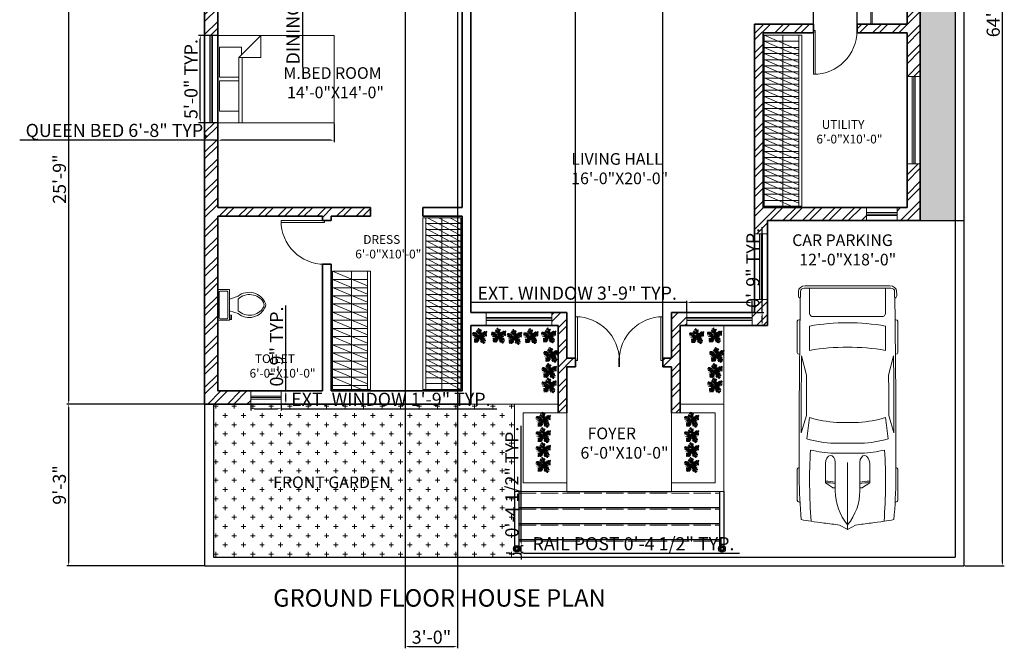
# Model space of a CAD drawing. Units: inches. Extents: x 108 to 883, y 608 to 1524.
# Tile 1 of 4: x 108 to 785, y 608 to 1040. Entities that reach past the tile are written whole.
import ezdxf

# ---------------------------------------------------------------- set-up
doc = ezdxf.new("R2010")
doc.units = ezdxf.units.IN
doc.linetypes.add('ACAD_ISO02W100', pattern=[15, 12, -3])
for name, color, linetype, lineweight in [('A-ANNO-DIMS', 2, 'Continuous', 18), ('A-ANNO-TEXT', 7, 'Continuous', 25), ('A-AREA-IDEN', 7, 'Continuous', 18), ('A-DOOR', 4, 'Continuous', 18), ('A-FLOR-CASE', 9, 'Continuous', 18), ('A-FLOR-CASE-HIDN', 9, 'ACAD_ISO02W100', 13), ('A-FLOR-CASE-PATT', 252, 'Continuous', 13), ('A-FLOR-FIXT', 9, 'Continuous', 18), ('A-FLOR-STRS', 7, 'Continuous', 25), ('A-FLOR-STRS-HIDN', 8, 'ACAD_ISO02W100', 13), ('A-FURN', 8, 'Continuous', 18), ('A-WALL', 7, 'Continuous', 35), ('A-WALL-PATT', 252, 'Continuous', 13), ('C-PKNG-VEHI', 8, 'Continuous', 13), ('C-PROP', 7, 'Continuous', 25), ('L-PLNT', 94, 'Continuous', 13), ('L-PLNT-BEDS', 94, 'Continuous', 18)]:
    doc.layers.add(name, color=color, linetype=linetype, lineweight=lineweight)
doc.layers.add('A-GLAZ', color=244, linetype='Continuous', lineweight=18, true_color=0x991b1e)
doc.layers.add('L-PLNT-PATT', color=116, linetype='Continuous', lineweight=13, true_color=0x136734)
doc.styles.get("Standard").update_dxf_attribs({"font": 'arial.ttf'})
doc.dimstyles.new('ISO-25', dxfattribs={"dimtxt": 9, "dimasz": 2.5, "dimexe": 1.25, "dimexo": 0.625, "dimtad": 1, "dimlunit": 3, "dimtxsty": 'Standard', "dimcen": 2.5, "dimadec": 0, "dimazin": 0, "dimtfac": 1, "dimtmove": 0, "dimatfit": 3, "dimfxl": 1, "dimarcsym": 0})

# ---------------------------------------------------------------- blocks, each defined once
blk = doc.blocks.new('*U2')
for p, q in [((0, 0), (0, -6)), ((40, 0), (40, -6))]:
    blk.add_line(p, q)
blk.add_lwpolyline([(0, 0), (0, 40), (1.75, 40), (1.75, 0)], close=True)
blk.add_arc((0, 0), 40, 0, 90)
blk = doc.blocks.new('*U4')
for p, q in [((0, 0), (0, -6)), ((-40, 0), (-40, -6))]:
    blk.add_line(p, q)
blk.add_lwpolyline([(0, 0), (0, 40), (-1.75, 40), (-1.75, 0)], close=True)
blk.add_arc((0, 0), 40, 90, 180)
blk = doc.blocks.new('*U7')
for p, q in [((46.55, 38.89), (22.35, 38.89)), ((136.7, 38.89), (160.9, 38.89)), ((21.1, 37.41), (21.1, 36.83)), ((47.8, 37.39), (47.8, 37.41)), ((70.03, 31.54), (86.41, 29.35)), ((87.99, 31.87), (74.76, 35.92)), ((134.31, 35.6), (119.29, 31.78)), ((135.45, 37.07), (135.45, 37.41)), ((162.15, 37.41), (162.15, 36.77)), ((186.47, -33.5), (186.47, 33.5)), ((188.4, -32.76), (188.4, 32.76)), ((138.42, 29.35), (157.25, 29.35)), ((164.52, 26.39), (164.52, -26.39)), ((186.47, 29.35), (167.01, 29.35)), ((32.27, 11.63), (36.13, 17.17)), ((36.13, 17.17), (50.94, 17.17)), ((29.77, 9.51), (51.68, 9.51)), ((32.12, 9.51), (32.12, 11.15)), ((58.92, -10.77), (58.92, 10.77)), ((66.55, -10.53), (66.55, 10.53)), ((82.74, 8.5), (82.74, -8.5)), ((186.47, -10.53), (186.47, 10.53)), ((3.27, 6.13), (0.1, 0.41)), ((0, 0), (51.68, 0)), ((0.1, -0.41), (3.27, -6.13)), ((29.77, -9.51), (51.68, -9.51)), ((32.12, -9.51), (32.12, -11.15)), ((32.27, -11.63), (36.13, -17.17)), ((36.13, -17.17), (50.94, -17.17)), ((86.41, -29.35), (70.03, -31.54)), ((157.25, -29.35), (138.42, -29.35)), ((167.01, -29.35), (186.47, -29.35)), ((21.1, -37.41), (21.1, -36.83)), ((47.8, -37.39), (47.8, -37.41)), ((87.99, -31.87), (74.76, -35.92)), ((134.31, -35.6), (119.29, -31.78)), ((135.45, -37.07), (135.45, -37.41)), ((162.15, -37.41), (162.15, -36.77)), ((46.55, -38.89), (22.35, -38.89)), ((136.7, -38.89), (160.9, -38.89))]:
    blk.add_line(p, q)
for centre, major_axis, ratio, start_param, end_param in [((22.35, 37.41), (0, -1.48), 0.842304, 3.141593, 4.712389), ((46.55, 37.41), (0, 1.48), 0.842304, -1.570796, 0), ((136.7, 37.41), (0, -1.48), 0.842304, 3.141593, 4.712389), ((160.9, 37.41), (0, 1.48), 0.842304, -1.570796, 0), ((266.03, -27.52), (0, 313.31), 0.842304, 1.367076, 1.39176), ((41.19, -490.86), (0, 528.23), 0.842304, 0.00281, 0.075598), ((64.48, -10555.62), (0, 10593.03), 0.842304, -0.013397, 0.002797), ((135.29, 5.39), (0, 81.77), 0.842304, 1.245306, 1.50788), ((64.48, -10555.62), (0, -10591.55), 0.842304, 3.133765, 3.140441), ((95.79, -3666.35), (0, -3698.24), 0.842304, 3.134049, 3.144098), ((180.63, 35.84), (0, 2.22), 0.842304, -0.013017, 1.249894), ((64.48, -10556.36), (0, 10595.31), 0.842304, -0.013397, -0.013017), ((183.98, 33.5), (0, -2.96), 0.842304, 1.570796, 3.128196), ((183.98, 32.76), (0, -5.25), 0.842304, 1.570796, 3.128196), ((259.18, -27.52), (0, -305.3), 0.842304, 4.528606, 4.561838), ((37.47, -593.96), (0, -623.33), 0.842304, 3.096046, 3.200911), ((134.4, 5.39), (0, -89.78), 0.842304, 4.449482, 4.652344), ((149.6, 2.8), (0, -79.58), 0.842304, 4.372215, 4.640744), ((17.08, 0), (0, 147.02), 0.842304, 4.511394, 4.913384), ((35.91, 0), (0, 147.02), 0.842304, 4.511394, 4.913384), ((167.01, 26.39), (0, 2.96), 0.842304, 0, 1.570796), ((-204.49, 52.4), (0, -250.96), 0.842304, 1.385369, 1.434372), ((13.04, 17.01), (0, 27.42), 0.842304, 4.435146, 4.718221), ((14.2, 17.01), (0, 27.42), 0.842304, 4.435146, 4.718221), ((50.79, 13.34), (6.34, -0.36), 0.603834, -1.395552, 1.581315), ((29.77, -46.66), (0, 56.17), 0.842304, 0, 0.590319), ((32.75, 11.15), (0, 0.74), 0.842304, 0.879714, 1.570796), ((0.62, 0), (0, -0.74), 0.842304, 4.131459, 5.293319), ((-204.49, -52.4), (0, 250.96), 0.842304, -1.434372, -1.385369), ((29.77, 46.66), (0, 56.17), 0.842304, 2.551274, 3.141593), ((32.75, -11.15), (0, -0.74), 0.842304, 4.712389, 5.403472), ((13.04, -17.01), (0, -27.42), 0.842304, 1.564964, 1.848039), ((14.2, -17.01), (0, -27.42), 0.842304, 1.564964, 1.848039), ((134.4, -5.39), (0, -89.78), 0.842304, -1.510751, -1.307889), ((135.29, -5.39), (0, -81.77), 0.842304, -1.50788, -1.245306), ((149.6, -2.8), (0, -79.58), 0.842304, -1.499151, -1.230623), ((259.18, 27.52), (0, 305.3), 0.842304, 1.721348, 1.754579), ((266.03, 27.52), (0, 313.31), 0.842304, 1.749832, 1.774517), ((37.47, 593.96), (0, -623.33), 0.842304, -0.059319, 0.045547), ((167.01, -26.39), (0, -2.96), 0.842304, 4.712389, 6.283185), ((41.19, 490.86), (0, -528.23), 0.842304, -0.075598, -0.00281), ((22.35, -37.41), (0, 1.48), 0.842304, 1.570796, 3.141593), ((64.48, 10555.62), (0, 10593.03), 0.842304, 3.138796, 3.15499), ((46.55, -37.41), (0, -1.48), 0.842304, 0, 1.570796), ((64.48, 10555.62), (0, -10591.55), 0.842304, 0.001152, 0.007828), ((95.79, 3666.35), (0, -3698.24), 0.842304, -0.002505, 0.007544), ((136.7, -37.41), (0, -1.48), 0.842304, -1.570796, 0), ((160.9, -37.41), (0, 1.48), 0.842304, 3.141593, 4.712389), ((180.63, -35.84), (0, -2.22), 0.842304, -1.249894, 0.013017), ((64.48, 10556.36), (0, 10595.31), 0.842304, 3.15461, 3.15499), ((183.98, -33.5), (0, 2.96), 0.842304, 3.15499, 4.712389), ((183.98, -32.76), (0, -5.25), 0.842304, 0.013397, 1.570796)]:
    blk.add_ellipse(centre, major_axis=major_axis, ratio=ratio, start_param=start_param, end_param=end_param)
at = {"extrusion": (0, 0, -1)}
blk.add_ellipse((50.79, -13.34), major_axis=(6.34, 0.36), ratio=0.603834, start_param=-1.395552, end_param=1.581315, dxfattribs=at)
blk = doc.blocks.new('*U9')
for p, q in [((9.5, -6), (9.5, -2)), ((-10, -8.5), (-8, -8.5)), ((-10, -9.5), (-10, -8.5)), ((-7, -9.5), (-10, -9.5)), ((-8, -8.5), (-8, -8)), ((-7, -8), (-7, -9.5)), ((-4, -8), (-6, -14)), ((4, -8), (6, -14)), ((4, -14), (-4, -14))]:
    blk.add_line(p, q)
blk.add_lwpolyline([(10.5, -8), (10.5, 0), (-10.5, 0), (-10.5, -8)], close=True)
for points in [[(-9.5, -2), (-9.5, -6)], [(8.5, -1), (-8.5, -1)], [(-8.5, -7), (8.5, -7)]]:
    blk.add_lwpolyline(points)
for centre, radius, start, end in [((-8.62, -1.88), 0.884, 81.8699, 188.1301), ((-8.62, -6.12), 0.884, 171.8699, 278.1301), ((8.62, -1.88), 0.884, 351.8699, 98.1301), ((8.62, -6.12), 0.884, 261.8699, 8.1301), ((3.52, -21.58), 12.17, 141.46911, 247.97143), ((4.2, -21.82), 11.33, 136.36773, 238.94682), ((-3.52, -21.58), 12.17, 292.02843, 38.53071), ((-4.2, -21.82), 11.33, 301.05301, 43.63209), ((0, -27.88), 4, 245.73182, 294.26817), ((0, -29), 4, 254.86053, 285.13947)]:
    blk.add_arc(centre, radius, start, end)
blk = doc.blocks.new('Bed - Queen')
for p, q in [((0, -80.00003), (0, 0)), ((0, 0), (59.99999, 0)), ((59.99999, 0), (59.99999, -80.00003)), ((7.99999, -1.2), (28.79998, -1.2)), ((7.99999, -14.4), (7.99999, -1.2)), ((28.79998, -1.2), (28.79998, -14.4)), ((31.19999, -1.2), (51.99999, -1.2)), ((31.19999, -14.4), (31.19999, -1.2)), ((51.99999, -1.2), (51.99999, -16.4)), ((0, -14.4), (44.8, -14.4)), ((44.8, -16.8), (0, -16.8)), ((59.99999, -29.6), (44.8, -14.4)), ((44.8, -14.4), (44.8, -29.6)), ((51.99999, -16.4), (46.79936, -16.4)), ((44.8, -29.6), (59.99999, -29.6)), ((59.99999, -80.00003), (0, -80.00003))]:
    blk.add_line(p, q)
blk = doc.blocks.new('*D14')
at = {"layer": 'A-ANNO-DIMS', "color": 0, "lineweight": -2, "transparency": 16777216}
for p, q in [((757.75, 1442.18), (784.93, 1442.18)), ((783.68, 667.61), (783.68, 1439.68)), ((757.75, 665.11), (784.93, 665.11))]:
    blk.add_line(p, q, dxfattribs=at)
at = {"layer": 'A-ANNO-DIMS', "color": 0, "transparency": 16777216}
for points in [[(783.26, 1439.68), (784.09, 1439.68), (783.68, 1442.18)], [(783.26, 667.61), (784.09, 667.61), (783.68, 665.11)]]:
    blk.add_solid(points, dxfattribs=at)
at = {"layer": 'Defpoints', "color": 0, "transparency": 16777216}
for p in [(757.12, 1442.18), (783.68, 1442.18), (757.12, 665.11)]:
    blk.add_point(p, dxfattribs=at)
at = {"layer": 'A-ANNO-DIMS', "color": 0, "transparency": 16777216, "insert": (778.46, 1053.64), "char_height": 9, "attachment_point": 5, "rotation": 90}
blk.add_mtext('64\'-9.07"', dxfattribs=at)
blk = doc.blocks.new('*U13')
for p, q in [((-47.498, 19.737), (-55.83, 18.344)), ((-40.615, 13.7), (-55.105, 10.913)), ((-31.5, 4.5), (-52.5, 25.5)), ((-33.37, 6.269), (-52.207, 5.34)), ((-48.585, 21.131), (-49.309, 29.026)), ((-28.299, 3.483), (-47.86, -5.805)), ((-43.513, 28.561), (-42.427, 15.558)), ((-38.442, 26.239), (-34.819, 7.663)), ((-21.416, 3.018), (-38.079, -8.128)), ((-35.544, 28.097), (-24.314, 3.947)), ((0, 0), (-31.5, 4.5)), ((-14.533, 2.09), (-30.834, 25.31)), ((-15.982, 2.09), (-30.11, -9.521)), ((-3.665, 19.273), (-27.574, 35.527)), ((-5.114, 28.097), (-24.676, 40.636)), ((-24.314, 23.917), (-2.941, 13.7)), ((0, 0), (-22.5, -19.5)), ((-7.288, 39.707), (-21.778, 46.673)), ((-6.563, 1.161), (-21.416, -8.128)), ((-20.691, 13.7), (-1.129, 4.876)), ((-8.737, 47.138), (-17.069, 52.711)), ((-10.186, 53.64), (-13.084, 55.962)), ((0, 0), (-10.5, 57)), ((-9.099, 51.782), (-6.563, 55.962)), ((-7.65, 43.423), (-2.578, 49.46)), ((-5.839, 35.992), (4.667, 48.067)), ((-5.114, 27.632), (10.463, 46.673)), ((-2.941, 16.486), (8.652, 37.85)), ((-1.129, 6.734), (9.014, 26.704)), ((0, 0), (27, 9)), ((0, 0), (18, -22.5)), ((3.942, 1.625), (11.187, 24.381)), ((6.478, 1.625), (26.04, -8.592)), ((10.101, 3.483), (17.708, 26.239)), ((11.187, 3.483), (30.749, -5.805)), ((16.259, 5.805), (23.142, 31.348)), ((18.07, 5.805), (35.096, -3.483)), ((22.055, 7.198), (27.489, 32.277)), ((24.229, 7.663), (46.688, 1.625)), ((27, 9), (48, 36)), ((27.127, 9.056), (31.112, 35.992)), ((29.662, 12.307), (48.137, 6.269)), ((31.836, 30.883), (32.561, 16.486)), ((33.285, 16.486), (48.862, 10.913)), ((35.096, 32.741), (37.27, 22.524)), ((36.183, 19.737), (48.137, 17.88)), ((38.719, 34.134), (41.979, 28.561)), ((40.53, 25.775), (48.862, 24.846)), ((43.791, 29.954), (51.036, 30.883)), ((44.153, 36.456), (45.239, 32.741)), ((-17.431, -15.094), (-42.789, -18.809)), ((-28.299, -29.026), (-42.789, -31.348)), ((-24.314, -21.596), (-42.427, -22.06)), ((-30.834, -34.135), (-42.427, -35.528)), ((-34.457, -39.708), (-40.978, -42.494)), ((-26.849, -26.24), (-40.253, -25.775)), ((-22.5, -19.5), (-37.5, -45)), ((-32.646, -36.921), (-31.921, -44.352)), ((-15.257, -12.772), (-30.11, -12.772)), ((-29.023, -30.884), (-27.936, -43.887)), ((-25.038, -23.918), (-22.865, -45.281)), ((-20.691, -18.345), (-17.793, -44.352)), ((-6.563, -5.805), (-19.967, -9.985)), ((-17.069, -15.094), (-12.721, -40.172)), ((-13.446, -11.378), (-8.737, -32.741)), ((-9.461, -8.592), (-6.201, -23.453)), ((-4.752, -3.483), (-3.665, -14.629)), ((2.493, -3.019), (-1.491, -20.202)), ((1.769, -2.555), (24.229, -9.521)), ((5.029, -6.27), (2.131, -25.775)), ((9.014, -11.378), (3.58, -35.992)), ((14.085, -16.951), (6.478, -40.172)), ((7.565, -9.056), (32.198, -14.629)), ((18.07, -22.524), (8.289, -45.745)), ((12.274, -15.094), (36.907, -18.809)), ((20.244, -30.419), (15.897, -44.816)), ((16.259, -19.738), (36.183, -22.989)), ((18, -22.5), (27, -52.5)), ((18.433, -22.524), (40.53, -29.026)), ((19.157, -25.311), (38.719, -33.206)), ((22.78, -37.85), (19.519, -48.532)), ((21.331, -32.741), (39.081, -40.636)), ((22.78, -38.314), (34.372, -44.816)), ((24.591, -45.745), (23.142, -50.854)), ((24.591, -43.423), (30.749, -47.603)), ((26.764, -49.925), (28.213, -50.854))]:
    blk.add_line(p, q)
blk = doc.blocks.new('WIN-45IN-EXT')
for p, q in [((3.5, 45), (3.5, 0)), ((4.5, 45), (4.5, 0)), ((5.5, 45), (5.5, 0))]:
    blk.add_line(p, q)
blk.add_lwpolyline([(9, 45), (9, 0), (0, 0), (0, 45)], close=True)
blk = doc.blocks.new('WIN-60IN-EXT')
for p, q in [((60, 5.5), (0, 5.5)), ((60, 4.5), (0, 4.5)), ((60, 3.5), (0, 3.5))]:
    blk.add_line(p, q)
blk.add_lwpolyline([(60, 9), (60, 0), (0, 0), (0, 9)], close=True)
blk = doc.blocks.new('WIN-21IN-EXT')
for p, q in [((0, 5.5), (21, 5.5)), ((0, 4.5), (21, 4.5)), ((0, 3.5), (21, 3.5))]:
    blk.add_line(p, q)
blk.add_lwpolyline([(0, 9), (21, 9), (21, 0), (0, 0)], close=True)
blk = doc.blocks.new('STAIR-RAIL-POST')
for radius in [2.29, 1.69, 1.09]:
    blk.add_circle((2.28, 2.28), radius)
blk = doc.blocks.new('*D28')
at = {"layer": 'A-ANNO-DIMS', "color": 0, "lineweight": -2, "transparency": 16777216}
for p, q in [((566.67, 839.8), (566.67, 847.18)), ((611.67, 839.8), (611.67, 847.18)), ((566.67, 845.93), (418.44, 845.93)), ((609.17, 845.93), (569.17, 845.93))]:
    blk.add_line(p, q, dxfattribs=at)
at = {"layer": 'A-ANNO-DIMS', "color": 0, "transparency": 16777216}
for points in [[(569.17, 846.34), (569.17, 845.51), (566.67, 845.93)], [(609.17, 846.34), (609.17, 845.51), (611.67, 845.93)]]:
    blk.add_solid(points, dxfattribs=at)
at = {"layer": 'Defpoints', "color": 0, "transparency": 16777216}
for p in [(566.67, 845.93), (566.67, 839.18), (611.67, 839.18)]:
    blk.add_point(p, dxfattribs=at)
at = {"layer": 'A-ANNO-DIMS', "color": 0, "transparency": 16777216, "insert": (491.3, 851.21), "char_height": 9, "attachment_point": 5}
blk.add_mtext('EXT. WINDOW 3\'-9" TYP.', dxfattribs=at)
blk = doc.blocks.new('*D29')
at = {"layer": 'A-ANNO-DIMS', "color": 0, "lineweight": -2, "transparency": 16777216}
for p, q in [((618.42, 839.18), (618.42, 897.79)), ((612.3, 839.18), (619.67, 839.18)), ((618.42, 832.68), (618.42, 836.68)), ((612.3, 830.18), (619.67, 830.18))]:
    blk.add_line(p, q, dxfattribs=at)
at = {"layer": 'A-ANNO-DIMS', "color": 0, "transparency": 16777216}
for points in [[(618, 836.68), (618.84, 836.68), (618.42, 839.18)], [(618, 832.68), (618.84, 832.68), (618.42, 830.18)]]:
    blk.add_solid(points, dxfattribs=at)
at = {"layer": 'Defpoints', "color": 0, "transparency": 16777216}
for p in [(611.67, 839.18), (618.42, 839.18), (611.67, 830.18)]:
    blk.add_point(p, dxfattribs=at)
at = {"layer": 'A-ANNO-DIMS', "color": 0, "transparency": 16777216, "insert": (613.2, 869.73), "char_height": 9, "attachment_point": 5, "rotation": 90}
blk.add_mtext('0\'-9" TYP.', dxfattribs=at)
blk = doc.blocks.new('*D30')
at = {"layer": 'A-ANNO-DIMS', "color": 0, "lineweight": -2, "transparency": 16777216}
for p, q in [((266.89, 775.55), (266.89, 771.78)), ((269.39, 773.03), (285.39, 773.03)), ((287.89, 775.55), (287.89, 771.78)), ((287.89, 773.03), (436.12, 773.03))]:
    blk.add_line(p, q, dxfattribs=at)
at = {"layer": 'A-ANNO-DIMS', "color": 0, "transparency": 16777216}
for points in [[(269.39, 773.44), (269.39, 772.61), (266.89, 773.03)], [(285.39, 773.44), (285.39, 772.61), (287.89, 773.03)]]:
    blk.add_solid(points, dxfattribs=at)
at = {"layer": 'Defpoints', "color": 0, "transparency": 16777216}
for p in [(266.89, 776.18), (287.89, 776.18), (287.89, 773.03)]:
    blk.add_point(p, dxfattribs=at)
at = {"layer": 'A-ANNO-DIMS', "color": 0, "transparency": 16777216, "insert": (363.25, 778.31), "char_height": 9, "attachment_point": 5}
blk.add_mtext('EXT. WINDOW 1\'-9" TYP.', dxfattribs=at)
blk = doc.blocks.new('*D31')
at = {"layer": 'A-ANNO-DIMS', "color": 0, "lineweight": -2, "transparency": 16777216}
for p, q in [((291.04, 785.18), (291.04, 843.79)), ((288.51, 785.18), (292.29, 785.18)), ((291.04, 778.68), (291.04, 782.68)), ((288.51, 776.18), (292.29, 776.18))]:
    blk.add_line(p, q, dxfattribs=at)
at = {"layer": 'A-ANNO-DIMS', "color": 0, "transparency": 16777216}
for points in [[(290.62, 782.68), (291.45, 782.68), (291.04, 785.18)], [(290.62, 778.68), (291.45, 778.68), (291.04, 776.18)]]:
    blk.add_solid(points, dxfattribs=at)
at = {"layer": 'Defpoints', "color": 0, "transparency": 16777216}
for p in [(287.89, 785.18), (291.04, 785.18), (287.89, 776.18)]:
    blk.add_point(p, dxfattribs=at)
at = {"layer": 'A-ANNO-DIMS', "color": 0, "transparency": 16777216, "insert": (285.82, 815.73), "char_height": 9, "attachment_point": 5, "rotation": 90}
blk.add_mtext('0\'-9" TYP.', dxfattribs=at)
blk = doc.blocks.new('*D34')
at = {"layer": 'A-ANNO-DIMS', "color": 0, "lineweight": -2, "transparency": 16777216}
for p, q in [((244.21, 968.8), (244.21, 956.17)), ((324.21, 968.8), (324.21, 956.17)), ((244.21, 957.42), (108.07, 957.42)), ((321.71, 957.42), (246.71, 957.42))]:
    blk.add_line(p, q, dxfattribs=at)
at = {"layer": 'A-ANNO-DIMS', "color": 0, "transparency": 16777216}
for points in [[(246.71, 957.84), (246.71, 957.01), (244.21, 957.42)], [(321.71, 957.84), (321.71, 957.01), (324.21, 957.42)]]:
    blk.add_solid(points, dxfattribs=at)
at = {"layer": 'Defpoints', "color": 0, "transparency": 16777216}
for p in [(244.21, 969.42), (324.21, 969.42), (244.21, 957.42)]:
    blk.add_point(p, dxfattribs=at)
at = {"layer": 'A-ANNO-DIMS', "color": 0, "transparency": 16777216, "insert": (174.89, 962.98), "char_height": 9, "attachment_point": 5}
blk.add_mtext('QUEEN BED 6\'-8" TYP.', dxfattribs=at)
blk = doc.blocks.new('*D35')
at = {"layer": 'A-ANNO-DIMS', "color": 0, "lineweight": -2, "transparency": 16777216}
for p, q in [((243.59, 1029.42), (230.96, 1029.42)), ((232.21, 971.92), (232.21, 1026.92)), ((243.59, 969.42), (230.96, 969.42))]:
    blk.add_line(p, q, dxfattribs=at)
at = {"layer": 'A-ANNO-DIMS', "color": 0, "transparency": 16777216}
for points in [[(231.8, 1026.92), (232.63, 1026.92), (232.21, 1029.42)], [(231.8, 971.92), (232.63, 971.92), (232.21, 969.42)]]:
    blk.add_solid(points, dxfattribs=at)
at = {"layer": 'Defpoints', "color": 0, "transparency": 16777216}
for p in [(232.21, 1029.42), (244.21, 1029.42), (244.21, 969.42)]:
    blk.add_point(p, dxfattribs=at)
at = {"layer": 'A-ANNO-DIMS', "color": 0, "transparency": 16777216, "insert": (226.99, 999.42), "char_height": 9, "attachment_point": 5, "rotation": 90}
blk.add_mtext('5\'-0" TYP.', dxfattribs=at)
blk = doc.blocks.new('*D36')
at = {"layer": 'A-ANNO-DIMS', "color": 0, "lineweight": -2, "transparency": 16777216}
for p, q in [((445.06, 673.83), (442.56, 673.83)), ((447.56, 673.89), (447.56, 672.58)), ((447.56, 673.83), (452.13, 673.83)), ((452.13, 673.89), (452.13, 672.58)), ((454.63, 673.83), (602.92, 673.83))]:
    blk.add_line(p, q, dxfattribs=at)
at = {"layer": 'A-ANNO-DIMS', "color": 0, "transparency": 16777216}
for points in [[(445.06, 674.25), (445.06, 673.42), (447.56, 673.83)], [(454.63, 674.25), (454.63, 673.42), (452.13, 673.83)]]:
    blk.add_solid(points, dxfattribs=at)
at = {"layer": 'Defpoints', "color": 0, "transparency": 16777216}
for p in [(447.56, 674.52), (452.13, 674.52), (452.13, 673.83)]:
    blk.add_point(p, dxfattribs=at)
at = {"layer": 'A-ANNO-DIMS', "color": 0, "transparency": 16777216, "insert": (530.03, 679.12), "char_height": 9, "attachment_point": 5}
blk.add_mtext('RAIL POST 0\'-4 1/2" TYP.', dxfattribs=at)
blk = doc.blocks.new('*D37')
at = {"layer": 'A-ANNO-DIMS', "color": 0, "lineweight": -2, "transparency": 16777216}
for p, q in [((452.82, 681.59), (452.82, 761.17)), ((452.76, 679.09), (454.07, 679.09)), ((452.82, 674.52), (452.82, 679.09)), ((452.76, 674.52), (454.07, 674.52)), ((452.82, 672.02), (452.82, 669.52))]:
    blk.add_line(p, q, dxfattribs=at)
at = {"layer": 'A-ANNO-DIMS', "color": 0, "transparency": 16777216}
for points in [[(452.4, 681.59), (453.24, 681.59), (452.82, 679.09)], [(452.4, 672.02), (453.24, 672.02), (452.82, 674.52)]]:
    blk.add_solid(points, dxfattribs=at)
at = {"layer": 'Defpoints', "color": 0, "transparency": 16777216}
for p in [(452.13, 679.09), (452.82, 679.09), (452.13, 674.52)]:
    blk.add_point(p, dxfattribs=at)
at = {"layer": 'A-ANNO-DIMS', "color": 0, "transparency": 16777216, "insert": (447.54, 722.63), "char_height": 9, "attachment_point": 5, "rotation": 90}
blk.add_mtext('0\'-4 1/2" TYP.', dxfattribs=at)
blk = doc.blocks.new('*D42')
at = {"layer": 'A-ANNO-DIMS', "color": 0, "lineweight": -2, "transparency": 16777216}
for p, q in [((315.42, 1201.24), (301.14, 1201.24)), ((302.39, 1198.74), (302.39, 1112.74)), ((315.42, 1110.24), (301.14, 1110.24)), ((302.39, 1110.24), (302.39, 1007.57))]:
    blk.add_line(p, q, dxfattribs=at)
at = {"layer": 'A-ANNO-DIMS', "color": 0, "transparency": 16777216}
for points in [[(301.98, 1198.74), (302.81, 1198.74), (302.39, 1201.24)], [(301.98, 1112.74), (302.81, 1112.74), (302.39, 1110.24)]]:
    blk.add_solid(points, dxfattribs=at)
at = {"layer": 'Defpoints', "color": 0, "transparency": 16777216}
for p in [(316.04, 1201.24), (302.39, 1110.24), (316.04, 1110.24)]:
    blk.add_point(p, dxfattribs=at)
at = {"layer": 'A-ANNO-DIMS', "color": 0, "transparency": 16777216, "insert": (297.11, 1057.66), "char_height": 9, "attachment_point": 5, "rotation": 90}
blk.add_mtext('DINING SET 7\'-7"', dxfattribs=at)
blk = doc.blocks.new('*D48')
at = {"layer": 'A-ANNO-DIMS', "color": 0, "lineweight": -2, "transparency": 16777216}
for p, q in [((234.59, 776.18), (140.51, 776.18)), ((141.76, 667.61), (141.76, 773.68)), ((234.59, 665.11), (140.51, 665.11))]:
    blk.add_line(p, q, dxfattribs=at)
at = {"layer": 'A-ANNO-DIMS', "color": 0, "transparency": 16777216}
for points in [[(141.35, 773.68), (142.18, 773.68), (141.76, 776.18)], [(141.35, 667.61), (142.18, 667.61), (141.76, 665.11)]]:
    blk.add_solid(points, dxfattribs=at)
at = {"layer": 'Defpoints', "color": 0, "transparency": 16777216}
for p in [(141.76, 776.18), (235.21, 776.18), (235.21, 665.11)]:
    blk.add_point(p, dxfattribs=at)
at = {"layer": 'A-ANNO-DIMS', "color": 0, "transparency": 16777216, "insert": (136.54, 720.64), "char_height": 9, "attachment_point": 5, "rotation": 90}
blk.add_mtext('9\'-3"', dxfattribs=at)
blk = doc.blocks.new('*D49')
at = {"layer": 'A-ANNO-DIMS', "color": 0, "lineweight": -2, "transparency": 16777216}
for p, q in [((234.59, 1085.18), (140.51, 1085.18)), ((141.76, 778.68), (141.76, 1082.68)), ((234.59, 776.18), (140.51, 776.18))]:
    blk.add_line(p, q, dxfattribs=at)
at = {"layer": 'A-ANNO-DIMS', "color": 0, "transparency": 16777216}
for points in [[(141.35, 1082.68), (142.18, 1082.68), (141.76, 1085.18)], [(141.35, 778.68), (142.18, 778.68), (141.76, 776.18)]]:
    blk.add_solid(points, dxfattribs=at)
at = {"layer": 'Defpoints', "color": 0, "transparency": 16777216}
for p in [(141.76, 1085.18), (235.21, 1085.18), (235.21, 776.18)]:
    blk.add_point(p, dxfattribs=at)
at = {"layer": 'A-ANNO-DIMS', "color": 0, "transparency": 16777216, "insert": (136.54, 930.68), "char_height": 9, "attachment_point": 5, "rotation": 90}
blk.add_mtext('25\'-9"', dxfattribs=at)
blk = doc.blocks.new('*D51')
at = {"layer": 'A-ANNO-DIMS', "color": 0, "lineweight": -2, "transparency": 16777216}
for p, q in [((373.12, 1078.55), (373.12, 608.47)), ((409.12, 1078.55), (409.12, 608.47)), ((375.62, 609.72), (406.62, 609.72))]:
    blk.add_line(p, q, dxfattribs=at)
at = {"layer": 'A-ANNO-DIMS', "color": 0, "transparency": 16777216}
for points in [[(375.62, 610.13), (375.62, 609.3), (373.12, 609.72)], [(406.62, 610.13), (406.62, 609.3), (409.12, 609.72)]]:
    blk.add_solid(points, dxfattribs=at)
at = {"layer": 'Defpoints', "color": 0, "transparency": 16777216}
for p in [(373.12, 1079.18), (409.12, 1079.18), (409.12, 609.72)]:
    blk.add_point(p, dxfattribs=at)
at = {"layer": 'A-ANNO-DIMS', "color": 0, "transparency": 16777216, "insert": (391.12, 614.94), "char_height": 9, "attachment_point": 5}
blk.add_mtext('3\'-0"', dxfattribs=at)
blk = doc.blocks.new('*D52')
at = {"layer": 'A-ANNO-DIMS', "color": 0, "lineweight": -2, "transparency": 16777216}
for p, q in [((653.67, 1031.8), (653.67, 1506.88)), ((656.17, 1505.63), (681.17, 1505.63)), ((683.67, 1031.8), (683.67, 1506.88))]:
    blk.add_line(p, q, dxfattribs=at)
at = {"layer": 'A-ANNO-DIMS', "color": 0, "transparency": 16777216}
for points in [[(656.17, 1506.04), (656.17, 1505.21), (653.67, 1505.63)], [(681.17, 1506.04), (681.17, 1505.21), (683.67, 1505.63)]]:
    blk.add_solid(points, dxfattribs=at)
at = {"layer": 'Defpoints', "color": 0, "transparency": 16777216}
for p in [(683.67, 1505.63), (653.67, 1031.18), (683.67, 1031.18)]:
    blk.add_point(p, dxfattribs=at)
at = {"layer": 'A-ANNO-DIMS', "color": 0, "transparency": 16777216, "insert": (668.67, 1510.85), "char_height": 9, "attachment_point": 5}
blk.add_mtext('2\'-6"', dxfattribs=at)
blk = doc.blocks.new('*D53')
at = {"layer": 'A-ANNO-DIMS', "color": 0, "lineweight": -2, "transparency": 16777216}
for p, q in [((490.21, 802.3), (490.21, 1506.88)), ((492.71, 1505.63), (547.71, 1505.63)), ((550.21, 802.3), (550.21, 1506.88))]:
    blk.add_line(p, q, dxfattribs=at)
at = {"layer": 'A-ANNO-DIMS', "color": 0, "transparency": 16777216}
for points in [[(492.71, 1506.04), (492.71, 1505.21), (490.21, 1505.63)], [(547.71, 1506.04), (547.71, 1505.21), (550.21, 1505.63)]]:
    blk.add_solid(points, dxfattribs=at)
at = {"layer": 'Defpoints', "color": 0, "transparency": 16777216}
for p in [(550.21, 1505.63), (490.21, 801.68), (550.21, 801.68)]:
    blk.add_point(p, dxfattribs=at)
at = {"layer": 'A-ANNO-DIMS', "color": 0, "transparency": 16777216, "insert": (520.21, 1510.85), "char_height": 9, "attachment_point": 5}
blk.add_mtext('5\'-0"', dxfattribs=at)

msp = doc.modelspace()

# ---------------------------------------------------------------- hatches: boundary and pattern name
at = {"layer": 'A-FLOR-CASE-PATT'}
h = msp.add_hatch(dxfattribs=at)
h.set_pattern_fill('ANSI31', color=256, scale=1.217335, angle=111.8141, style=0)
h.paths.add_polyline_path([(632.527, 912.177), (643.767, 912.177), (643.767, 1021.211), (624.184, 1029.598), (619.767, 1029.598), (619.767, 917.642)])
h = msp.add_hatch(dxfattribs=at)
h.set_pattern_fill('ANSI31', color=256, scale=1.323525, angle=-45, style=0)
h.paths.add_polyline_path([(643.767, 913.433), (643.767, 1027.279), (619.767, 1027.279), (619.767, 913.433)])
h = msp.add_hatch(dxfattribs=at)
h.set_pattern_fill('ANSI31', color=256, scale=1.13134, angle=106.948, style=0)
h.paths.add_polyline_path([(407.775, 786.177), (411.212, 786.177), (411.212, 902.034), (407.191, 904.177), (387.212, 904.177), (387.212, 797.134)])
h = msp.add_hatch(dxfattribs=at)
h.set_pattern_fill('ANSI31', color=256, scale=1.28295, angle=-45, style=0)
h.paths.add_polyline_path([(411.212, 788.416), (411.212, 902.036), (387.212, 902.036), (387.212, 788.416)])
h = msp.add_hatch(dxfattribs=at)
h.set_pattern_fill('ANSI31', color=256, scale=1.627438, angle=112.3196, style=0)
h.paths.add_polyline_path([(337.07, 786.177), (347.212, 786.177), (347.212, 859.917), (329.242, 867.427), (323.212, 867.427), (323.212, 791.968)])
h = msp.add_hatch(dxfattribs=at)
h.set_pattern_fill('ANSI31', color=256, scale=1.76239, angle=-45, style=0)
h.paths.add_polyline_path([(347.212, 786.36), (347.212, 864.334), (323.212, 864.334), (323.212, 786.36)])
at = {"layer": 'A-WALL-PATT'}
h = msp.add_hatch(dxfattribs=at)
h.set_pattern_fill('ANSI32', color=256)
h.paths.add_polyline_path([(373.121, 1085.177), (292.121, 1085.177), (292.121, 1127.011), (283.121, 1127.011), (283.121, 1085.177), (235.212, 1085.177), (235.212, 1029.423), (244.212, 1029.423), (244.212, 1079.177), (373.121, 1079.177), (373.121, 1084.577)])
h.paths.add_polyline_path([(349.212, 911.177), (244.212, 911.177), (244.212, 969.423), (235.212, 969.423), (235.212, 776.177), (266.885, 776.177), (266.885, 785.177), (244.212, 785.177), (244.212, 905.177), (316.212, 905.177), (316.212, 902.177), (322.212, 902.177), (322.212, 905.177), (349.212, 905.177)])
h.paths.add_polyline_path([(484.212, 839.177), (473.778, 839.177), (473.778, 830.177), (478.212, 830.177), (478.212, 770.177), (484.212, 770.177), (484.212, 801.677), (490.212, 801.677), (490.212, 806.177), (490.212, 807.677), (484.212, 807.677)])
h.paths.add_polyline_path([(562.212, 830.177), (566.671, 830.177), (566.671, 839.177), (556.212, 839.177), (556.212, 807.677), (550.212, 807.677), (550.212, 806.177), (550.212, 801.677), (556.212, 801.677), (556.212, 770.177), (562.212, 770.177)])
h.paths.add_polyline_path([(622.212, 848.109), (613.212, 848.109), (613.212, 839.177), (611.671, 839.177), (611.671, 830.177), (622.212, 830.177)])
h.paths.add_polyline_path([(690.201, 911.177), (619.212, 911.177), (619.212, 1031.177), (653.667, 1031.177), (653.667, 1037.177), (613.212, 1037.177), (613.212, 893.109), (622.212, 893.109), (622.212, 902.177), (690.201, 902.177)])
h.paths.add_polyline_path([(727.121, 941.177), (718.121, 941.177), (718.121, 911.177), (711.201, 911.177), (711.201, 902.177), (727.121, 902.177)])
h.paths.add_polyline_path([(727.121, 1103.177), (718.121, 1103.177), (718.121, 1037.177), (683.667, 1037.177), (683.667, 1031.177), (718.121, 1031.177), (718.121, 1001.177), (727.121, 1001.177)])
h.paths.add_polyline_path([(727.121, 1412.177), (676.121, 1412.177), (676.121, 1403.177), (718.121, 1403.177), (718.121, 1295.236), (727.121, 1295.236)])
h.paths.add_polyline_path([(574.121, 1403.177), (616.121, 1403.177), (616.121, 1412.177), (548.621, 1412.177), (548.621, 1403.177), (568.121, 1403.177), (568.121, 1307.177), (565.121, 1307.177), (565.121, 1301.177), (568.121, 1301.177), (568.121, 1274.177), (574.121, 1274.177)])
h.paths.add_polyline_path([(508.121, 1403.177), (527.621, 1403.177), (527.621, 1412.177), (483.029, 1412.177), (483.029, 1403.177), (502.121, 1403.177), (502.121, 1307.177), (475.121, 1307.177), (475.121, 1301.177), (535.121, 1301.177), (535.121, 1307.177), (508.121, 1307.177)])
h.paths.add_polyline_path([(462.029, 1412.177), (394.121, 1412.177), (394.121, 1403.177), (436.121, 1403.177), (436.121, 1274.177), (442.121, 1274.177), (442.121, 1301.177), (445.121, 1301.177), (445.121, 1307.177), (442.121, 1307.177), (442.121, 1403.177), (462.029, 1403.177)])
h.paths.add_polyline_path([(334.121, 1412.177), (283.121, 1412.177), (283.121, 1288.13), (292.121, 1288.13), (292.121, 1403.177), (334.121, 1403.177)])
at = {"layer": 'L-PLNT-PATT'}
h = msp.add_hatch(dxfattribs=at)
h.set_pattern_fill('CROSS', color=256)
h.paths.add_polyline_path([(751.121, 1436.177), (241.212, 1436.177), (241.212, 1085.177), (283.121, 1085.177), (283.121, 1412.177), (727.121, 1412.177), (727.121, 902.177), (751.121, 902.177)])
h = msp.add_hatch(dxfattribs=at)
h.set_pattern_fill('CROSS', color=256)
h.paths.add_polyline_path([(449.849, 671.11), (449.849, 674.52, -0.4142136), (447.564, 676.805, -0.1955108), (448.212, 678.399), (448.212, 716.11), (448.212, 776.177), (418.212, 776.177), (241.212, 776.177), (241.212, 671.11)])
h.paths.add_polyline_path([(279.413, 713.941), (372.821, 713.941), (372.821, 730.426), (279.413, 730.426)], flags=24)

# ---------------------------------------------------------------- linework, layer by layer
at = {"layer": 'A-FLOR-CASE'}
for p, q in [((694.121, 1229.177), (694.121, 1037.177)), ((619.767, 1029.598), (619.767, 912.177)), ((619.767, 1029.598), (645.767, 1029.598)), ((632.767, 912.177), (632.767, 1029.598)), ((643.767, 1029.598), (643.767, 912.177)), ((645.767, 1029.598), (645.767, 912.177)), ((619.767, 912.177), (645.767, 912.177)), ((385.212, 904.177), (385.212, 786.177)), ((385.212, 904.177), (411.212, 904.177)), ((387.212, 904.177), (387.212, 786.177)), ((398.212, 904.177), (398.212, 786.177)), ((411.212, 904.177), (411.212, 786.177)), ((323.212, 867.427), (323.212, 786.177)), ((323.212, 867.427), (349.212, 867.427)), ((336.212, 786.177), (336.212, 867.427)), ((347.212, 867.427), (347.212, 786.177)), ((349.212, 867.427), (349.212, 786.177)), ((323.212, 786.177), (349.212, 786.177)), ((385.212, 786.177), (411.212, 786.177))]:
    msp.add_line(p, q, dxfattribs=at)
at = {"layer": 'A-FLOR-CASE-HIDN'}
msp.add_line((693.121, 1229.177), (693.121, 1037.177), dxfattribs=at)
at = {"layer": 'A-FLOR-STRS'}
for p, q in [((448.212, 716.11), (448.212, 678.399)), ((451.212, 716.11), (451.212, 678.639)), ((484.212, 716.11), (556.212, 716.11)), ((589.212, 716.11), (589.212, 678.399)), ((592.212, 716.11), (592.212, 678.639)), ((451.212, 705.11), (589.212, 705.11)), ((451.212, 694.11), (589.212, 694.11)), ((451.212, 683.11), (589.212, 683.11))]:
    msp.add_line(p, q, dxfattribs=at)
at = {"layer": 'A-FLOR-STRS-HIDN'}
for p, q in [((451.212, 715.11), (589.212, 715.11)), ((451.212, 704.11), (589.212, 704.11)), ((451.212, 693.11), (589.212, 693.11)), ((451.212, 682.11), (589.212, 682.11))]:
    msp.add_line(p, q, dxfattribs=at)
at = {"layer": 'A-WALL'}
for p, q in [((727.121, 1412.177), (727.121, 902.177)), ((718.121, 1229.177), (718.121, 1037.177)), ((235.212, 1085.177), (235.212, 776.177)), ((244.212, 1079.177), (244.212, 911.177)), ((412.212, 1079.177), (412.212, 911.177)), ((418.212, 1079.177), (418.212, 839.177)), ((613.212, 1037.177), (613.212, 839.177)), ((613.212, 1037.177), (653.667, 1037.177)), ((653.667, 1031.177), (653.667, 1037.177)), ((683.667, 1031.177), (683.667, 1037.177)), ((683.667, 1037.177), (718.121, 1037.177)), ((619.212, 1031.177), (653.667, 1031.177)), ((619.212, 1031.177), (619.212, 911.177)), ((683.667, 1031.177), (718.121, 1031.177)), ((718.121, 1031.177), (718.121, 911.177)), ((244.212, 911.177), (349.212, 911.177)), ((349.212, 905.177), (349.212, 911.177)), ((385.212, 905.177), (385.212, 911.177)), ((385.212, 911.177), (412.212, 911.177)), ((619.212, 911.177), (718.121, 911.177)), ((244.212, 905.177), (316.212, 905.177)), ((244.212, 905.177), (244.212, 785.177)), ((316.212, 905.177), (316.212, 902.177)), ((322.212, 902.177), (316.212, 902.177)), ((322.212, 905.177), (322.212, 902.177)), ((322.212, 905.177), (349.212, 905.177)), ((385.212, 905.177), (412.212, 905.177)), ((412.212, 905.177), (412.212, 785.177)), ((622.212, 902.177), (727.121, 902.177)), ((622.212, 902.177), (622.212, 830.177)), ((322.212, 872.177), (316.212, 872.177)), ((316.212, 872.177), (316.212, 785.177)), ((322.212, 872.177), (322.212, 785.177)), ((418.212, 839.177), (484.212, 839.177)), ((484.212, 807.677), (484.212, 839.177)), ((556.212, 839.177), (613.212, 839.177)), ((556.212, 807.677), (556.212, 839.177)), ((418.212, 830.177), (478.212, 830.177)), ((418.212, 830.177), (418.212, 776.177)), ((478.212, 770.177), (478.212, 830.177)), ((562.212, 770.177), (562.212, 830.177)), ((562.212, 830.177), (622.212, 830.177)), ((484.212, 807.677), (490.212, 807.677)), ((490.212, 801.677), (490.212, 807.677)), ((520.212, 801.677), (520.212, 807.677)), ((550.212, 801.677), (550.212, 807.677)), ((550.212, 807.677), (556.212, 807.677)), ((484.212, 770.177), (484.212, 801.677)), ((484.212, 801.677), (490.212, 801.677)), ((550.212, 801.677), (556.212, 801.677)), ((556.212, 770.177), (556.212, 801.677)), ((244.212, 785.177), (316.212, 785.177)), ((322.212, 785.177), (412.212, 785.177)), ((235.212, 776.177), (418.212, 776.177))]:
    msp.add_line(p, q, dxfattribs=at)
at = {"layer": 'C-PROP'}
for p, q in [((757.121, 1442.177), (757.121, 665.11)), ((751.121, 1436.177), (751.121, 671.11)), ((727.121, 902.177), (757.121, 902.177)), ((235.212, 776.177), (235.212, 665.11)), ((241.212, 776.177), (241.212, 671.11)), ((241.212, 671.11), (751.121, 671.11)), ((235.212, 665.11), (757.121, 665.11))]:
    msp.add_line(p, q, dxfattribs=at)
at = {"layer": 'L-PLNT-BEDS'}
for p, q in [((592.212, 830.177), (592.212, 716.11)), ((418.212, 776.177), (448.212, 776.177)), ((478.212, 776.177), (448.212, 776.177)), ((448.212, 776.177), (448.212, 716.11)), ((562.212, 776.177), (592.212, 776.177)), ((454.212, 770.177), (454.212, 722.11)), ((484.212, 770.177), (454.212, 770.177)), ((484.212, 722.11), (484.212, 770.177)), ((556.212, 770.177), (586.212, 770.177)), ((556.212, 722.11), (556.212, 770.177)), ((586.212, 770.177), (586.212, 722.11)), ((454.212, 722.11), (484.212, 722.11)), ((484.212, 722.11), (484.212, 716.11)), ((556.212, 722.11), (556.212, 716.11)), ((556.212, 722.11), (586.212, 722.11)), ((448.212, 716.11), (484.212, 716.11)), ((556.212, 716.11), (592.212, 716.11))]:
    msp.add_line(p, q, dxfattribs=at)

# ---------------------------------------------------------------- block references
at = {"layer": 'A-DOOR', "xscale": 0.7499760613271671, "yscale": 0.7499760613271671, "zscale": 0.7499760613271671}
for p, rotation in [((653.667, 1032.677), 180), ((317.712, 902.177), 89.99999999999996)]:
    msp.add_blockref('*U4', p, dxfattribs=dict(at, rotation=rotation))
at = {"layer": 'A-DOOR', "yscale": 0.75, "zscale": 0.75}
for p, xscale in [((490.212, 806.177), 0.75), ((550.212, 806.177), -0.75)]:
    msp.add_blockref('*U2', p, dxfattribs=dict(at, xscale=xscale))
at = {"layer": 'A-FLOR-FIXT', "rotation": 90}
msp.add_blockref('*U9', (244.212, 844.299), dxfattribs=at)
at = {"layer": 'A-FLOR-STRS'}
for p in [(447.564, 674.52), (588.564, 674.52)]:
    msp.add_blockref('STAIR-RAIL-POST', p, dxfattribs=at)
at = {"layer": 'A-FURN', "rotation": 90}
msp.add_blockref('Bed - Queen', (244.212, 969.423), dxfattribs=at)
at = {"layer": 'A-GLAZ', "rotation": 90}
for name, p in [('WIN-60IN-EXT', (244.212, 969.423)), ('WIN-60IN-EXT', (727.121, 941.176)), ('WIN-45IN-EXT', (473.778, 830.177)), ('WIN-45IN-EXT', (611.672, 830.177))]:
    msp.add_blockref(name, p, dxfattribs=at)
at = {"layer": 'A-GLAZ'}
for name, p in [('WIN-21IN-EXT', (690.201, 902.177)), ('WIN-45IN-EXT', (613.212, 848.109)), ('WIN-21IN-EXT', (266.885, 776.177))]:
    msp.add_blockref(name, p, dxfattribs=at)
at = {"layer": 'C-PKNG-VEHI', "xscale": 0.8882973855907836, "yscale": 0.8882973855907836, "zscale": 0.8882973855907836, "rotation": 90}
msp.add_blockref('*U7', (677.163, 690.117), dxfattribs=at)
at = {"layer": 'L-PLNT', "xscale": 0.0967505621858107, "yscale": 0.0967505621858107, "zscale": 0.0967505621858107}
for p in [(424.568, 822.753), (437.536, 822.967), (448.436, 822.05), (459.746, 822.598), (471.982, 823.061), (573.746, 822.598), (585.982, 823.061), (473.568, 809.717), (587.568, 809.717), (472.368, 798.694), (586.368, 798.694), (472.254, 788.777), (586.254, 788.777), (468.306, 765.11), (570.306, 765.11), (468.306, 754.592), (570.306, 754.592), (468.306, 744.374), (570.306, 744.374), (468.306, 734.156), (570.306, 734.156)]:
    msp.add_blockref('*U13', p, dxfattribs=at)

# ---------------------------------------------------------------- texts
at = {"layer": 'A-ANNO-TEXT', "insert": (282.33, 649.055), "char_height": 12, "attachment_point": 1}
msp.add_mtext_dynamic_manual_height_columns('GROUND FLOOR HOUSE PLAN ', width=283.6624, gutter_width=12.5, heights=[0], dxfattribs=at)
at = {"layer": 'A-AREA-IDEN', "attachment_point": 1}
for s, width, insert, char_height in [('M.BED ROOM\\P 14\'-0"X14\'-0"', 78.97922, (289.429, 1007.568), 8), ('  UTILITY \\P6\'-0"X10\'-0"', 43.83658, (655.753, 971.184), 6), ('LIVING HALL\\P16\'-0"X20\'-0"', 67.22379, (487.248, 948.546), 8), ('   DRESS \\P6\'-0"X10\'-0"', 43.83658, (338.769, 892.239), 6), ('CAR PARKING\\P  12\'-0"X18\'-0"', 77.00568, (639.13, 892.766), 8), ('  TOILET \\P6\'-0"X10\'-0"', 43.83658, (266.073, 810.37), 6), ('  FOYER\\P6\'-0"X10\'-0"', 58.43074, (493.572, 760.047), 8), ('FRONT GARDEN', 89.74024, (282.33, 726.451), 8)]:
    msp.add_mtext_dynamic_manual_height_columns(s, width=width, gutter_width=12.5, heights=[0], dxfattribs=dict(at, insert=insert, char_height=char_height))

# ---------------------------------------------------------------- dimensions: what is measured, and where the dimension line sits
at = {"layer": 'A-ANNO-DIMS'}
for base, p1, p2, picture, middle in [((550.212, 1505.627), (490.212, 801.677), (550.212, 801.677), '*D53', (520.212, 1510.847)), ((683.667, 1505.627), (653.667, 1031.177), (683.667, 1031.177), '*D52', (668.667, 1510.847)), ((409.121, 609.715), (373.121, 1079.177), (409.121, 1079.177), '*D51', (391.121, 614.938))]:
    dim = msp.add_linear_dim(base=base, p1=p1, p2=p2, dimstyle='ISO-25', override={"dimdec": 1, "dimlfac": 1, "dimrnd": 0, "dimzin": 1, "dimdsep": 46, "dimlunit": 4, "dimfrac": 2}, dxfattribs=at)
    dim.commit()
    dim.dimension.update_dxf_attribs({"geometry": picture, "text_midpoint": middle})
for base, p1, p2, override, picture, middle in [((783.676, 1442.177), (757.121, 665.11), (757.121, 1442.177), {"dimclrd": 0, "dimclre": 0, "dimclrt": 0}, '*D14', (778.456, 1053.644)), ((141.762, 1085.177), (235.212, 776.177), (235.212, 1085.177), {"dimdec": 1, "dimlfac": 1, "dimrnd": 0, "dimzin": 1, "dimdsep": 46, "dimlunit": 4, "dimfrac": 2}, '*D49', (136.542, 930.677)), ((141.762, 776.177), (235.212, 665.11), (235.212, 776.177), {"dimdec": 1, "dimlfac": 1, "dimrnd": 0, "dimzin": 1, "dimdsep": 46, "dimlunit": 4, "dimfrac": 2}, '*D48', (136.539, 720.644))]:
    dim = msp.add_linear_dim(base=base, p1=p1, p2=p2, angle=90, dimstyle='ISO-25', override=override, dxfattribs=at)
    dim.commit()
    dim.dimension.update_dxf_attribs({"geometry": picture, "text_midpoint": middle})
for base, p1, p2, angle, text, picture, middle in [((302.393, 1110.242), (316.043, 1201.242), (316.043, 1110.242), 270, 'DINING SET <>', '*D42', (297.114, 1057.657)), ((232.212, 1029.423), (244.212, 969.423), (244.212, 1029.423), 90, '<> TYP.', '*D35', (226.992, 999.423)), ((244.212, 957.423), (324.212, 969.423), (244.212, 969.423), 180, 'QUEEN BED <> TYP.', '*D34', (174.891, 962.978)), ((618.421, 839.177), (611.671, 830.177), (611.671, 839.177), 90, '<> TYP.', '*D29', (613.201, 869.732)), ((566.671, 845.927), (611.671, 839.177), (566.671, 839.177), 180, 'EXT. WINDOW <> TYP.', '*D28', (491.304, 851.211)), ((291.035, 785.177), (287.885, 776.177), (287.885, 785.177), 90, '<> TYP.', '*D31', (285.815, 815.732)), ((452.819, 679.09), (452.134, 674.52), (452.134, 679.09), 90, '<> TYP.', '*D37', (447.541, 722.63))]:
    dim = msp.add_linear_dim(base=base, p1=p1, p2=p2, angle=angle, text=text, dimstyle='ISO-25', override={"dimdec": 1, "dimlfac": 1, "dimrnd": 0, "dimzin": 1, "dimdsep": 46, "dimlunit": 4, "dimfrac": 2}, dxfattribs=at)
    dim.commit()
    dim.dimension.update_dxf_attribs({"geometry": picture, "text_midpoint": middle})
for base, p1, p2, text, picture, middle in [((287.885, 773.027), (266.885, 776.177), (287.885, 776.177), 'EXT. WINDOW <> TYP.', '*D30', (363.253, 778.308)), ((452.134, 673.834), (447.564, 674.52), (452.134, 674.52), 'RAIL POST <> TYP.', '*D36', (530.026, 679.116))]:
    dim = msp.add_linear_dim(base=base, p1=p1, p2=p2, text=text, dimstyle='ISO-25', override={"dimdec": 1, "dimlfac": 1, "dimrnd": 0, "dimzin": 1, "dimdsep": 46, "dimlunit": 4, "dimfrac": 2}, dxfattribs=at)
    dim.commit()
    dim.dimension.update_dxf_attribs({"geometry": picture, "text_midpoint": middle})

doc.saveas('drawing.dxf')
